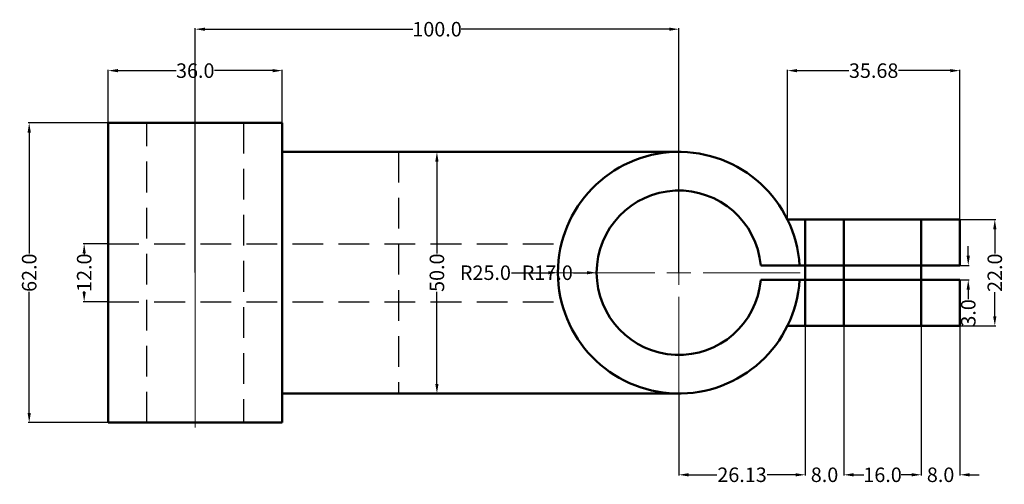
# Model space of a CAD drawing. Units: inches. Extents: x 196 to 456, y 125 to 440.
# Tile 2 of 2: x 253 to 456, y 344 to 440. Entities that reach past the tile are written whole.
import ezdxf

# ---------------------------------------------------------------- set-up
doc = ezdxf.new("R2010")
doc.units = ezdxf.units.IN
doc.header["$MEASUREMENT"] = 0
doc.linetypes.add('CENTER', pattern=[50.8, 31.75, -6.35, 6.35, -6.35])
doc.linetypes.add('HIDDEN', pattern=[9.525, 6.35, -3.175])
for name, color, linetype, lineweight in [('M-CNTR', 1, 'CENTER', 18), ('M-DIMS', 2, 'Continuous', 25), ('M-HIDN', 6, 'HIDDEN', 25), ('M-OUTL', 7, 'Continuous', 50)]:
    doc.layers.add(name, color=color, linetype=linetype, lineweight=lineweight)
doc.styles.get("Standard").update_dxf_attribs({"font": 'arial.ttf'})
doc.dimstyles.get("Standard").update_dxf_attribs({"dimtxt": 3, "dimasz": 2, "dimexe": 0.18, "dimexo": 0.0625, "dimgap": 0.09, "dimtad": 0, "dimdec": 1, "dimzin": 0, "dimdsep": 46, "dimtxsty": 'Standard', "dimcen": 0.09, "dimadec": 0, "dimazin": 0, "dimtfac": 1, "dimtdec": 1, "dimtofl": 0, "dimtmove": 0, "dimatfit": 3, "dimfxl": 1, "dimtolj": 1, "dimtzin": 0, "dimarcsym": 0})

# ---------------------------------------------------------------- blocks, each defined once
blk = doc.blocks.new('*U1')
at = {"layer": 'M-CNTR', "color": 0, "transparency": 16777216}
for p, q in [((0, 5), (0, 25.12)), ((-25.12, 0), (-5, 0)), ((5, 0), (25.12, 0)), ((0, -25.12), (0, -5))]:
    blk.add_line(p, q, dxfattribs=at)
at = {"layer": 'M-CNTR', "color": 0, "linetype": 'Continuous', "transparency": 16777216}
for p, q in [((0, -2.5), (0, 2.5)), ((-2.5, 0), (2.5, 0))]:
    blk.add_line(p, q, dxfattribs=at)
blk = doc.blocks.new('*U5')
at = {"layer": 'M-CNTR', "color": 0, "ltscale": 8, "transparency": 16777216}
blk.add_line((0, -32), (0, 32), dxfattribs=at)
blk = doc.blocks.new('*D6')
at = {"layer": 'Defpoints', "color": 0, "transparency": 16777216}
for p in [(447.1, 398.76), (454.31, 398.76), (447.1, 376.76)]:
    blk.add_point(p, dxfattribs=at)
at = {"layer": 'M-DIMS', "color": 0, "lineweight": -2, "transparency": 16777216}
for p, q in [((447.16, 398.76), (454.49, 398.76)), ((454.31, 396.76), (454.31, 391.76)), ((454.31, 378.76), (454.31, 383.75)), ((447.16, 376.76), (454.49, 376.76))]:
    blk.add_line(p, q, dxfattribs=at)
at = {"layer": 'M-DIMS', "color": 0, "transparency": 16777216}
for points in [[(453.97, 396.76), (454.64, 396.76), (454.31, 398.76)], [(453.97, 378.76), (454.64, 378.76), (454.31, 376.76)]]:
    blk.add_solid(points, dxfattribs=at)
at = {"layer": 'M-DIMS', "color": 0, "transparency": 16777216, "insert": (454.31, 387.76), "char_height": 3, "attachment_point": 5, "rotation": 90}
blk.add_mtext('\\A1;22.0', dxfattribs=at)
blk = doc.blocks.new('*D7')
at = {"layer": 'Defpoints', "color": 0, "transparency": 16777216}
for p in [(288.97, 438.13), (288.97, 387.76), (388.97, 387.76)]:
    blk.add_point(p, dxfattribs=at)
at = {"layer": 'M-DIMS', "color": 0, "lineweight": -2, "transparency": 16777216}
for p, q in [((288.97, 387.82), (288.97, 438.31)), ((290.97, 438.13), (333.97, 438.13)), ((386.97, 438.13), (343.98, 438.13)), ((388.97, 387.82), (388.97, 438.31))]:
    blk.add_line(p, q, dxfattribs=at)
at = {"layer": 'M-DIMS', "color": 0, "transparency": 16777216}
for points in [[(290.97, 438.46), (290.97, 437.8), (288.97, 438.13)], [(386.97, 438.46), (386.97, 437.8), (388.97, 438.13)]]:
    blk.add_solid(points, dxfattribs=at)
at = {"layer": 'M-DIMS', "color": 0, "transparency": 16777216, "insert": (338.97, 438.13), "char_height": 3, "attachment_point": 5}
blk.add_mtext('\\A1;100.0', dxfattribs=at)
blk = doc.blocks.new('*D8')
at = {"layer": 'Defpoints', "color": 0, "transparency": 16777216}
for p in [(270.97, 393.76), (266, 381.76), (270.97, 381.76)]:
    blk.add_point(p, dxfattribs=at)
at = {"layer": 'M-DIMS', "color": 0, "lineweight": -2, "transparency": 16777216}
for p, q in [((270.91, 393.76), (265.82, 393.76)), ((266, 391.76), (266, 391.6)), ((266, 383.76), (266, 383.92)), ((270.91, 381.76), (265.82, 381.76))]:
    blk.add_line(p, q, dxfattribs=at)
at = {"layer": 'M-DIMS', "color": 0, "transparency": 16777216}
for points in [[(265.67, 391.76), (266.33, 391.76), (266, 393.76)], [(265.67, 383.76), (266.33, 383.76), (266, 381.76)]]:
    blk.add_solid(points, dxfattribs=at)
at = {"layer": 'M-DIMS', "color": 0, "transparency": 16777216, "insert": (266, 387.76), "char_height": 3, "attachment_point": 5, "rotation": 90}
blk.add_mtext('\\A1;12.0', dxfattribs=at)
blk = doc.blocks.new('*D9')
at = {"layer": 'Defpoints', "color": 0, "transparency": 16777216}
for p in [(254.63, 418.76), (270.97, 418.76), (270.97, 356.76)]:
    blk.add_point(p, dxfattribs=at)
at = {"layer": 'M-DIMS', "color": 0, "lineweight": -2, "transparency": 16777216}
for p, q in [((270.91, 418.76), (254.45, 418.76)), ((254.63, 416.76), (254.63, 391.75)), ((254.63, 358.76), (254.63, 383.77)), ((270.91, 356.76), (254.45, 356.76))]:
    blk.add_line(p, q, dxfattribs=at)
at = {"layer": 'M-DIMS', "color": 0, "transparency": 16777216}
for points in [[(254.3, 416.76), (254.97, 416.76), (254.63, 418.76)], [(254.3, 358.76), (254.97, 358.76), (254.63, 356.76)]]:
    blk.add_solid(points, dxfattribs=at)
at = {"layer": 'M-DIMS', "color": 0, "transparency": 16777216, "insert": (254.63, 387.76), "char_height": 3, "attachment_point": 5, "rotation": 90}
blk.add_mtext('\\A1;62.0', dxfattribs=at)
blk = doc.blocks.new('*D10')
at = {"layer": 'Defpoints', "color": 0, "transparency": 16777216}
for p in [(347.97, 412.76), (338.94, 362.76), (347.97, 362.76)]:
    blk.add_point(p, dxfattribs=at)
at = {"layer": 'M-DIMS', "color": 0, "lineweight": -2, "transparency": 16777216}
for p, q in [((347.91, 412.76), (338.76, 412.76)), ((338.94, 410.76), (338.94, 391.74)), ((338.94, 364.76), (338.94, 383.78)), ((347.91, 362.76), (338.76, 362.76))]:
    blk.add_line(p, q, dxfattribs=at)
at = {"layer": 'M-DIMS', "color": 0, "transparency": 16777216}
for points in [[(338.61, 410.76), (339.27, 410.76), (338.94, 412.76)], [(338.61, 364.76), (339.27, 364.76), (338.94, 362.76)]]:
    blk.add_solid(points, dxfattribs=at)
at = {"layer": 'M-DIMS', "color": 0, "transparency": 16777216, "insert": (338.94, 387.76), "char_height": 3, "attachment_point": 5, "rotation": 90}
blk.add_mtext('\\A1;50.0', dxfattribs=at)
blk = doc.blocks.new('*D23')
at = {"layer": 'Defpoints', "color": 0, "transparency": 16777216}
for p in [(447.1, 389.26), (447.1, 386.26), (448.82, 386.26)]:
    blk.add_point(p, dxfattribs=at)
at = {"layer": 'M-DIMS', "color": 0, "lineweight": -2, "transparency": 16777216}
for p, q in [((448.82, 391.26), (448.82, 393.26)), ((447.16, 389.26), (449, 389.26)), ((447.16, 386.26), (449, 386.26)), ((448.82, 384.26), (448.82, 382.26))]:
    blk.add_line(p, q, dxfattribs=at)
at = {"layer": 'M-DIMS', "color": 0, "transparency": 16777216}
for points in [[(448.48, 391.26), (449.15, 391.26), (448.82, 389.26)], [(448.48, 384.26), (449.15, 384.26), (448.82, 386.26)]]:
    blk.add_solid(points, dxfattribs=at)
at = {"layer": 'M-DIMS', "color": 0, "transparency": 16777216, "insert": (448.82, 379.44), "char_height": 3, "attachment_point": 5, "rotation": 90}
blk.add_mtext('\\A1;3.0', dxfattribs=at)
blk = doc.blocks.new('*D31')
at = {"layer": 'Defpoints', "color": 0, "transparency": 16777216}
for p in [(306.97, 429.56), (270.97, 418.76), (306.97, 418.76)]:
    blk.add_point(p, dxfattribs=at)
at = {"layer": 'M-DIMS', "color": 0, "lineweight": -2, "transparency": 16777216}
for p, q in [((270.97, 418.82), (270.97, 429.74)), ((306.97, 418.82), (306.97, 429.74)), ((272.97, 429.56), (284.99, 429.56)), ((304.97, 429.56), (292.95, 429.56))]:
    blk.add_line(p, q, dxfattribs=at)
at = {"layer": 'M-DIMS', "color": 0, "transparency": 16777216}
for points in [[(272.97, 429.89), (272.97, 429.22), (270.97, 429.56)], [(304.97, 429.89), (304.97, 429.22), (306.97, 429.56)]]:
    blk.add_solid(points, dxfattribs=at)
at = {"layer": 'M-DIMS', "color": 0, "transparency": 16777216, "insert": (288.97, 429.56), "char_height": 3, "attachment_point": 5}
blk.add_mtext('\\A1;36.0', dxfattribs=at)
blk = doc.blocks.new('*D32')
at = {"layer": 'Defpoints', "color": 0, "transparency": 16777216}
for p in [(447.1, 429.56), (411.42, 398.76), (447.1, 398.76)]:
    blk.add_point(p, dxfattribs=at)
at = {"layer": 'M-DIMS', "color": 0, "lineweight": -2, "transparency": 16777216}
for p, q in [((411.42, 398.82), (411.42, 429.74)), ((447.1, 398.82), (447.1, 429.74)), ((413.42, 429.56), (424.11, 429.56)), ((445.1, 429.56), (434.42, 429.56))]:
    blk.add_line(p, q, dxfattribs=at)
at = {"layer": 'M-DIMS', "color": 0, "transparency": 16777216}
for points in [[(413.42, 429.89), (413.42, 429.22), (411.42, 429.56)], [(445.1, 429.89), (445.1, 429.22), (447.1, 429.56)]]:
    blk.add_solid(points, dxfattribs=at)
at = {"layer": 'M-DIMS', "color": 0, "transparency": 16777216, "insert": (429.26, 429.56), "char_height": 3, "attachment_point": 5}
blk.add_mtext('\\A1;35.68', dxfattribs=at)
blk = doc.blocks.new('*D33')
at = {"layer": 'Defpoints', "color": 0, "transparency": 16777216}
for p in [(415.1, 376.76), (388.97, 362.76), (415.1, 345.96)]:
    blk.add_point(p, dxfattribs=at)
at = {"layer": 'M-DIMS', "color": 0, "lineweight": -2, "transparency": 16777216}
for p, q in [((415.1, 376.69), (415.1, 345.78)), ((388.97, 362.69), (388.97, 345.78)), ((390.97, 345.96), (396.86, 345.96)), ((413.1, 345.96), (407.21, 345.96))]:
    blk.add_line(p, q, dxfattribs=at)
at = {"layer": 'M-DIMS', "color": 0, "transparency": 16777216}
for points in [[(390.97, 346.29), (390.97, 345.62), (388.97, 345.96)], [(413.1, 346.29), (413.1, 345.62), (415.1, 345.96)]]:
    blk.add_solid(points, dxfattribs=at)
at = {"layer": 'M-DIMS', "color": 0, "transparency": 16777216, "insert": (402.04, 345.96), "char_height": 3, "attachment_point": 5}
blk.add_mtext('\\A1;26.13', dxfattribs=at)
blk = doc.blocks.new('*D34')
at = {"layer": 'Defpoints', "color": 0, "transparency": 16777216}
for p in [(415.1, 376.76), (423.1, 376.76), (423.1, 345.96)]:
    blk.add_point(p, dxfattribs=at)
at = {"layer": 'M-DIMS', "color": 0, "lineweight": -2, "transparency": 16777216}
for p, q in [((415.1, 376.69), (415.1, 345.78)), ((423.1, 376.69), (423.1, 345.78)), ((413.1, 345.96), (411.1, 345.96)), ((425.1, 345.96), (427.1, 345.96))]:
    blk.add_line(p, q, dxfattribs=at)
at = {"layer": 'M-DIMS', "color": 0, "transparency": 16777216}
for points in [[(413.1, 346.29), (413.1, 345.62), (415.1, 345.96)], [(425.1, 346.29), (425.1, 345.62), (423.1, 345.96)]]:
    blk.add_solid(points, dxfattribs=at)
at = {"layer": 'M-DIMS', "color": 0, "transparency": 16777216, "insert": (419.1, 345.96), "char_height": 3, "attachment_point": 5}
blk.add_mtext('\\A1;8.0', dxfattribs=at)
blk = doc.blocks.new('*D35')
at = {"layer": 'Defpoints', "color": 0, "transparency": 16777216}
for p in [(423.1, 376.76), (439.1, 376.76), (439.1, 345.96)]:
    blk.add_point(p, dxfattribs=at)
at = {"layer": 'M-DIMS', "color": 0, "lineweight": -2, "transparency": 16777216}
for p, q in [((423.1, 376.69), (423.1, 345.78)), ((439.1, 376.69), (439.1, 345.78)), ((425.1, 345.96), (427.26, 345.96)), ((437.1, 345.96), (434.94, 345.96))]:
    blk.add_line(p, q, dxfattribs=at)
at = {"layer": 'M-DIMS', "color": 0, "transparency": 16777216}
for points in [[(425.1, 346.29), (425.1, 345.62), (423.1, 345.96)], [(437.1, 346.29), (437.1, 345.62), (439.1, 345.96)]]:
    blk.add_solid(points, dxfattribs=at)
at = {"layer": 'M-DIMS', "color": 0, "transparency": 16777216, "insert": (431.1, 345.96), "char_height": 3, "attachment_point": 5}
blk.add_mtext('\\A1;16.0', dxfattribs=at)
blk = doc.blocks.new('*D36')
at = {"layer": 'Defpoints', "color": 0, "transparency": 16777216}
for p in [(439.1, 376.76), (447.1, 376.76), (447.1, 345.96)]:
    blk.add_point(p, dxfattribs=at)
at = {"layer": 'M-DIMS', "color": 0, "lineweight": -2, "transparency": 16777216}
for p, q in [((439.1, 376.69), (439.1, 345.78)), ((447.1, 376.69), (447.1, 345.78)), ((437.1, 345.96), (435.1, 345.96)), ((449.1, 345.96), (451.1, 345.96))]:
    blk.add_line(p, q, dxfattribs=at)
at = {"layer": 'M-DIMS', "color": 0, "transparency": 16777216}
for points in [[(437.1, 346.29), (437.1, 345.62), (439.1, 345.96)], [(449.1, 346.29), (449.1, 345.62), (447.1, 345.96)]]:
    blk.add_solid(points, dxfattribs=at)
at = {"layer": 'M-DIMS', "color": 0, "transparency": 16777216, "insert": (443.1, 345.96), "char_height": 3, "attachment_point": 5}
blk.add_mtext('\\A1;8.0', dxfattribs=at)
blk = doc.blocks.new('*D42')
at = {"layer": 'Defpoints', "color": 0, "transparency": 16777216}
for p in [(363.97, 387.76), (388.97, 387.76)]:
    blk.add_point(p, dxfattribs=at)
at = {"layer": 'M-DIMS', "color": 0, "lineweight": -2, "transparency": 16777216}
for p, q in [((354.39, 387.76), (361.97, 387.76)), ((388.88, 387.76), (389.06, 387.76)), ((388.97, 387.67), (388.97, 387.85))]:
    blk.add_line(p, q, dxfattribs=at)
at = {"layer": 'M-DIMS', "color": 0, "transparency": 16777216}
blk.add_solid([(361.97, 388.09), (361.97, 387.42), (363.97, 387.76)], dxfattribs=at)
at = {"layer": 'M-DIMS', "color": 0, "transparency": 16777216, "insert": (348.97, 387.76), "char_height": 3, "attachment_point": 5, "rotation": 0.0008}
blk.add_mtext('\\A1;R25.0', dxfattribs=at)
blk = doc.blocks.new('*D43')
at = {"layer": 'Defpoints', "color": 0, "transparency": 16777216}
for p in [(371.97, 387.76), (388.97, 387.76)]:
    blk.add_point(p, dxfattribs=at)
at = {"layer": 'M-DIMS', "color": 0, "lineweight": -2, "transparency": 16777216}
for p, q in [((367.19, 387.76), (369.97, 387.76)), ((388.88, 387.76), (389.06, 387.76)), ((388.97, 387.67), (388.97, 387.85))]:
    blk.add_line(p, q, dxfattribs=at)
at = {"layer": 'M-DIMS', "color": 0, "transparency": 16777216}
blk.add_solid([(369.97, 388.09), (369.97, 387.42), (371.97, 387.76)], dxfattribs=at)
at = {"layer": 'M-DIMS', "color": 0, "transparency": 16777216, "insert": (361.77, 387.76), "char_height": 3, "attachment_point": 5, "rotation": 0.0012}
blk.add_mtext('\\A1;R17.0', dxfattribs=at)

msp = doc.modelspace()

# ---------------------------------------------------------------- linework, layer by layer
at = {"layer": 'M-HIDN'}
for p, q in [((278.973, 356.756), (278.973, 418.756)), ((298.973, 418.756), (298.973, 356.756)), ((330.973, 412.756), (330.973, 362.756)), ((270.973, 393.756), (364.703, 393.756)), ((270.973, 381.756), (364.703, 381.756))]:
    msp.add_line(p, q, dxfattribs=at)
at = {"layer": 'M-OUTL'}
for p, q in [((270.973, 356.756), (270.973, 418.756)), ((270.973, 418.756), (306.973, 418.756)), ((306.973, 418.756), (306.973, 356.756)), ((306.973, 412.756), (388.973, 412.756)), ((411.423, 398.756), (424.651, 398.756)), ((411.423, 398.756), (447.101, 398.756)), ((415.101, 398.756), (415.101, 376.756)), ((423.101, 398.756), (423.101, 376.756)), ((439.101, 398.756), (439.101, 376.756)), ((447.101, 398.756), (447.101, 389.256)), ((405.906, 389.256), (447.101, 389.256)), ((405.906, 386.256), (447.101, 386.256)), ((447.101, 386.256), (447.101, 376.756)), ((411.423, 376.756), (424.651, 376.756)), ((447.101, 376.756), (424.651, 376.756)), ((306.973, 362.756), (388.973, 362.756)), ((306.973, 356.756), (270.973, 356.756))]:
    msp.add_line(p, q, dxfattribs=at)
for radius, start, end in [(25, 3.43981, 356.56019), (17, 5.06209, 354.93791)]:
    msp.add_arc((388.973, 387.756), radius, start, end, dxfattribs=at)

# ---------------------------------------------------------------- block references
at = {"layer": 'M-CNTR', "ltscale": 8}
msp.add_blockref('*U5', (288.973, 387.756), dxfattribs=at)
at = {"layer": 'M-CNTR'}
msp.add_blockref('*U1', (388.973, 387.756), dxfattribs=at)

# ---------------------------------------------------------------- dimensions: what is measured, and where the dimension line sits
at = {"layer": 'M-DIMS'}
for base, p1, p2, override, picture, middle in [((288.973, 438.129), (388.973, 387.756), (288.973, 387.756), {"dimclrd": 0, "dimclre": 0, "dimclrt": 0}, '*D7', (338.973, 438.129)), ((306.973, 429.556), (270.973, 418.756), (306.973, 418.756), {"dimdec": 1, "dimlfac": 1, "dimrnd": 0, "dimzin": 0, "dimdsep": 46, "dimlunit": 2}, '*D31', (288.973, 429.556)), ((447.101, 429.556), (411.423, 398.756), (447.101, 398.756), {"dimdec": 2, "dimlfac": 1, "dimrnd": 0, "dimzin": 0, "dimdsep": 46, "dimlunit": 2}, '*D32', (429.262, 429.556)), ((415.101, 345.956), (388.973, 362.756), (415.101, 376.756), {"dimdec": 2, "dimlfac": 1, "dimrnd": 0, "dimzin": 0, "dimdsep": 46, "dimlunit": 2}, '*D33', (402.037, 345.956)), ((423.101, 345.956), (415.101, 376.756), (423.101, 376.756), {"dimdec": 1, "dimlfac": 1, "dimrnd": 0, "dimzin": 0, "dimdsep": 46, "dimlunit": 2}, '*D34', (419.101, 345.956)), ((439.101, 345.956), (423.101, 376.756), (439.101, 376.756), {"dimdec": 1, "dimlfac": 1, "dimrnd": 0, "dimzin": 0, "dimdsep": 46, "dimlunit": 2}, '*D35', (431.101, 345.956)), ((447.101, 345.956), (439.101, 376.756), (447.101, 376.756), {"dimdec": 1, "dimlfac": 1, "dimrnd": 0, "dimzin": 0, "dimdsep": 46, "dimlunit": 2}, '*D36', (443.101, 345.956))]:
    dim = msp.add_linear_dim(base=base, p1=p1, p2=p2, dimstyle='Standard', override=override, dxfattribs=at)
    dim.commit()
    dim.dimension.update_dxf_attribs({"geometry": picture, "text_midpoint": middle})
for base, p1, p2, picture, middle in [((254.632, 418.756), (270.973, 356.756), (270.973, 418.756), '*D9', (254.632, 387.756)), ((338.94, 362.756), (347.973, 412.756), (347.973, 362.756), '*D10', (338.94, 387.756)), ((454.306, 398.756), (447.101, 376.756), (447.101, 398.756), '*D6', (454.306, 387.756)), ((266, 381.756), (270.973, 393.756), (270.973, 381.756), '*D8', (266, 387.756)), ((448.815, 386.256), (447.101, 389.256), (447.101, 386.256), '*D23', (448.815, 379.442))]:
    dim = msp.add_linear_dim(base=base, p1=p1, p2=p2, angle=90, dimstyle='Standard', override={"dimclrd": 0, "dimclre": 0, "dimclrt": 0}, dxfattribs=at)
    dim.commit()
    dim.dimension.update_dxf_attribs({"geometry": picture, "text_midpoint": middle})
for mpoint, picture, middle in [((363.973, 387.756), '*D42', (348.973, 387.756)), ((371.973, 387.756), '*D43', (361.773, 387.756))]:
    dim = msp.add_radius_dim(center=(388.973, 387.756), mpoint=mpoint, dimstyle='Standard', override={"dimdec": 1, "dimlfac": 1, "dimrnd": 0, "dimzin": 0, "dimdsep": 46, "dimlunit": 2}, dxfattribs=at)
    dim.commit()
    dim.dimension.update_dxf_attribs({"geometry": picture, "text_midpoint": middle, "dimtype": 164})

doc.saveas('drawing.dxf')
